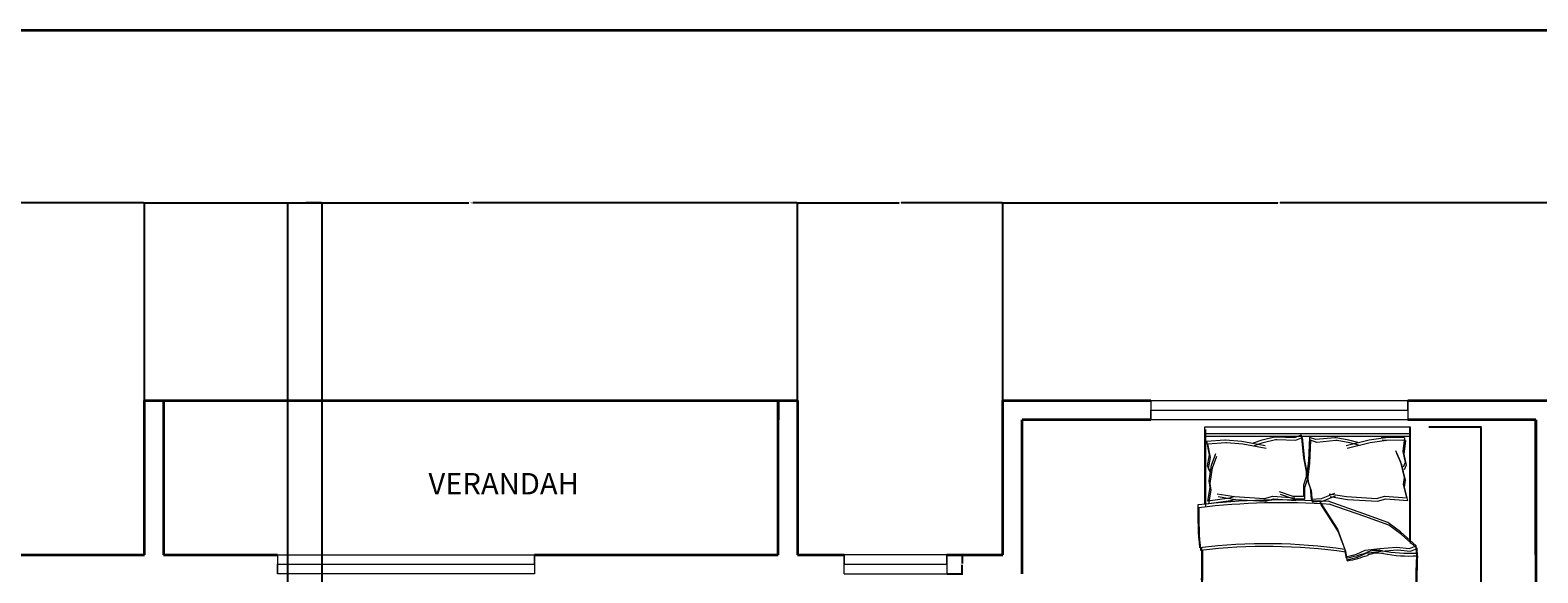
# Model space of a CAD drawing. Units: inches. Extents: x 1937 to 2996, y 1402 to 2323.
# Tile 8 of 10: x 2290 to 2643, y 2197 to 2323. Entities that reach past the tile are written whole.
import ezdxf

# ---------------------------------------------------------------- set-up
doc = ezdxf.new("R2010")
doc.units = ezdxf.units.IN
for name, color, linetype, lineweight in [('A-ANNO-DIMS', 2, 'Continuous', 18), ('A-ANNO-TTLB', 7, 'Continuous', 35), ('A-AREA-IDEN', 7, 'Continuous', 18), ('A-FURN', 8, 'Continuous', 13), ('A-GLAZ', 141, 'Continuous', 18), ('A-WALL', 7, 'Continuous', 35)]:
    doc.layers.add(name, color=color, linetype=linetype, lineweight=lineweight)
doc.styles.get("Standard").update_dxf_attribs({"font": 'arial.ttf'})
doc.dimstyles.get("Standard").update_dxf_attribs({"dimtxt": 0.18, "dimasz": 0.18, "dimexe": 0.18, "dimexo": 0.0625, "dimgap": 0.09, "dimtad": 0, "dimtih": 1, "dimtoh": 1, "dimdec": 4, "dimzin": 0, "dimdsep": 46, "dimtxsty": 'Standard', "dimcen": 0.09, "dimadec": 0, "dimazin": 0, "dimtfac": 1, "dimtdec": 4, "dimtofl": 0, "dimtmove": 0, "dimatfit": 3, "dimfxl": 1, "dimtolj": 1, "dimtzin": 0, "dimarcsym": 0})

# ---------------------------------------------------------------- blocks, each defined once
blk = doc.blocks.new('BED-DOUBLE')
for p, q in [((-24.01, -18.11), (-24.01, 0)), ((-24.01, -18.11), (-24.01, 0)), ((-24.01, 0), (24.01, 0)), ((23.78, 0), (23.78, -26.61)), ((23.78, 0), (23.78, -26.61)), ((24.01, 0), (24.01, -0.64)), ((-24.01, -1.53), (23.78, -1.53)), ((-24.01, -1.53), (23.78, -1.53)), ((-23.78, -18.75), (-23.78, -0.64)), ((-23.78, -18.75), (-23.78, -0.64)), ((-23.78, -2.17), (24.01, -2.17)), ((-23.78, -2.17), (24.01, -2.17)), ((-23.59, -3.34), (-19.3, -3.01)), ((-23.59, -3.34), (-19.31, -3.01)), ((-23.59, -3.32), (-23.01, -6.5)), ((-23.59, -3.32), (-23.01, -6.5)), ((-19.31, -3.01), (-19.2, -3.03)), ((-19.3, -3.01), (-19.2, -3.03)), ((-19.2, -3.03), (-15.38, -3.32)), ((-19.2, -3.03), (-15.38, -3.32)), ((-15.38, -3.32), (-9.88, -4.33)), ((-15.38, -3.32), (-9.88, -4.33)), ((-12.63, -3.75), (-10.61, -3.03)), ((-12.63, -3.75), (-10.61, -3.03)), ((-10.61, -3.03), (-7.71, -2.3)), ((-10.61, -3.03), (-7.71, -2.3)), ((-10.38, -3.67), (-7.49, -2.94)), ((-10.38, -3.67), (-7.49, -2.94)), ((-7.71, -2.3), (-7.39, -2.3)), ((-7.71, -2.3), (-7.39, -2.3)), ((-7.49, -2.94), (-7.16, -2.94)), ((-7.49, -2.94), (-7.16, -2.94)), ((-7.39, -2.3), (-2.95, -2.45)), ((-7.39, -2.3), (-2.95, -2.45)), ((-7.16, -2.94), (-2.72, -3.09)), ((-7.16, -2.94), (-2.72, -3.09)), ((-2.95, -2.45), (-1.5, -1.87)), ((-2.95, -2.45), (-1.5, -1.87)), ((-2.72, -3.09), (-1.27, -2.51)), ((-2.72, -3.09), (-1.27, -2.51)), ((-1.5, -1.87), (-0.92, -7.22)), ((-1.5, -1.87), (-0.92, -7.22)), ((-1.27, -2.51), (-0.7, -7.86)), ((-1.27, -2.51), (-0.7, -7.86)), ((0.49, -2.49), (0.25, -7.87)), ((0.49, -2.49), (0.25, -7.87)), ((0.72, -3.13), (0.48, -8.51)), ((0.72, -3.13), (0.48, -8.51)), ((1.97, -2.98), (0.49, -2.49)), ((1.97, -2.98), (0.49, -2.49)), ((2.2, -3.62), (0.72, -3.13)), ((2.2, -3.62), (0.72, -3.13)), ((6.4, -2.56), (1.97, -2.98)), ((6.4, -2.56), (1.97, -2.98)), ((6.63, -3.2), (2.2, -3.62)), ((6.63, -3.2), (2.2, -3.62)), ((6.72, -2.54), (6.4, -2.56)), ((6.72, -2.54), (6.4, -2.56)), ((6.95, -3.18), (6.63, -3.2)), ((6.95, -3.18), (6.63, -3.2)), ((9.65, -3.08), (6.72, -2.54)), ((9.65, -3.08), (6.72, -2.54)), ((9.88, -3.72), (6.95, -3.18)), ((9.88, -3.72), (6.95, -3.18)), ((14.43, -3.07), (9.01, -4.42)), ((14.43, -3.07), (9.01, -4.42)), ((11.72, -3.67), (9.65, -3.08)), ((11.72, -3.67), (9.65, -3.08)), ((18.23, -2.54), (14.43, -3.07)), ((18.23, -2.54), (14.43, -3.07)), ((18.46, -3.18), (14.66, -3.71)), ((18.46, -3.18), (14.66, -3.71)), ((22.63, -2.56), (17.23, -2.46)), ((17.23, -2.46), (18.23, -2.54)), ((22.63, -2.56), (17.23, -2.46)), ((17.23, -2.46), (18.23, -2.54)), ((22.86, -3.2), (17.45, -3.1)), ((17.45, -3.1), (18.46, -3.18)), ((22.86, -3.2), (17.45, -3.1)), ((17.45, -3.1), (18.46, -3.18)), ((22.63, -2.56), (22.25, -5.77)), ((22.63, -2.56), (22.25, -5.77)), ((22.86, -3.2), (22.48, -6.41)), ((22.86, -3.2), (22.48, -6.41)), ((24.01, -0.64), (24.01, -27.25)), ((24.01, -0.64), (24.01, -27.25)), ((-23.01, -6.5), (-23.45, -9.1)), ((-23.01, -6.5), (-23.45, -9.1)), ((-23.36, -3.98), (-19.08, -3.65)), ((-23.36, -3.98), (-19.08, -3.65)), ((-23.36, -3.96), (-22.78, -7.14)), ((-23.36, -3.96), (-22.78, -7.14)), ((-22.43, -8.96), (-21.42, -6.21)), ((-22.43, -8.96), (-21.42, -6.21)), ((-22.21, -9.59), (-21.19, -6.85)), ((-22.2, -9.59), (-21.19, -6.85)), ((-19.08, -3.65), (-18.97, -3.67)), ((-19.08, -3.65), (-18.97, -3.67)), ((-18.97, -3.67), (-15.15, -3.96)), ((-18.97, -3.67), (-15.15, -3.96)), ((-15.15, -3.96), (-9.65, -4.97)), ((-15.15, -3.96), (-9.65, -4.97)), ((-12.4, -4.39), (-10.38, -3.67)), ((-12.4, -4.39), (-10.38, -3.67)), ((14.66, -3.71), (9.24, -5.06)), ((14.66, -3.71), (9.24, -5.06)), ((11.94, -4.31), (9.88, -3.72)), ((11.94, -4.31), (9.88, -3.72)), ((21.83, -8.26), (20.64, -5.58)), ((21.82, -8.26), (20.64, -5.58)), ((22.05, -8.9), (20.87, -6.22)), ((22.05, -8.9), (20.87, -6.22)), ((22.25, -5.77), (22.84, -8.34)), ((22.25, -5.77), (22.84, -8.34)), ((22.48, -6.41), (23.07, -8.98)), ((22.48, -6.41), (23.07, -8.98)), ((-23.45, -9.1), (-22.87, -10.11)), ((-23.45, -9.1), (-22.87, -10.11)), ((-22.78, -7.14), (-23.22, -9.74)), ((-22.78, -7.14), (-23.22, -9.74)), ((-23.22, -9.74), (-22.64, -10.75)), ((-23.22, -9.74), (-22.64, -10.75)), ((-23.01, -12.57), (-22.43, -8.96)), ((-23.01, -12.57), (-22.43, -8.96)), ((-22.78, -13.21), (-22.2, -9.59)), ((-22.78, -13.21), (-22.21, -9.59)), ((-0.92, -7.22), (-0.35, -10.4)), ((-0.92, -7.22), (-0.35, -10.4)), ((-0.7, -7.86), (-0.12, -11.04)), ((-0.7, -7.86), (-0.12, -11.04)), ((-0.35, -10.4), (-0.35, -11.7)), ((-0.35, -10.4), (-0.35, -11.7)), ((0.25, -7.87), (-0.13, -11.08)), ((0.25, -7.87), (-0.13, -11.08)), ((0.48, -8.51), (0.1, -11.72)), ((0.48, -8.51), (0.1, -11.72)), ((22.63, -11.83), (21.82, -8.26)), ((22.63, -11.83), (21.83, -8.26)), ((22.86, -12.47), (22.05, -8.9)), ((22.86, -12.47), (22.05, -8.9)), ((22.84, -8.34), (22.33, -9.38)), ((22.84, -8.34), (22.33, -9.38)), ((23.07, -8.98), (22.56, -10.02)), ((23.07, -8.98), (22.56, -10.02)), ((-22.72, -14.16), (-23.01, -12.57)), ((-22.72, -14.16), (-23.01, -12.57)), ((-22.49, -14.8), (-22.78, -13.21)), ((-22.49, -14.8), (-22.78, -13.21)), ((-0.35, -11.7), (-0.92, -13.58)), ((-0.35, -11.7), (-0.92, -13.58)), ((-0.92, -13.58), (-0.92, -16.26)), ((-0.92, -13.58), (-0.92, -16.26)), ((-0.12, -12.34), (-0.7, -14.22)), ((-0.12, -12.34), (-0.7, -14.22)), ((-0.13, -11.08), (-0.05, -12.38)), ((-0.13, -11.08), (-0.05, -12.38)), ((-0.12, -11.04), (-0.12, -12.34)), ((-0.12, -11.04), (-0.12, -12.34)), ((-0.05, -12.38), (0.65, -14.22)), ((-0.05, -12.38), (0.65, -14.22)), ((0.1, -11.72), (0.18, -13.02)), ((0.1, -11.72), (0.18, -13.02)), ((0.18, -13.02), (0.87, -14.86)), ((0.18, -13.02), (0.87, -14.86)), ((22.44, -13.43), (22.63, -11.83)), ((22.44, -13.43), (22.63, -11.83)), ((23.21, -16.57), (22.44, -13.43)), ((23.21, -16.57), (22.44, -13.43)), ((22.67, -14.07), (22.86, -12.47)), ((22.67, -14.07), (22.86, -12.47)), ((23.44, -17.21), (22.67, -14.07)), ((23.44, -17.21), (22.67, -14.07)), ((-23.3, -17.34), (-22.72, -14.16)), ((-23.3, -17.34), (-22.72, -14.16)), ((-18.2, -16.62), (-23.3, -17.34)), ((-18.2, -16.62), (-23.3, -17.34)), ((-23.07, -17.98), (-22.49, -14.8)), ((-23.07, -17.98), (-22.49, -14.8)), ((-17.98, -17.26), (-23.07, -17.98)), ((-17.98, -17.26), (-23.07, -17.98)), ((-21.1, -15.63), (-17.07, -16.3)), ((-21.1, -15.63), (-17.07, -16.3)), ((-20.87, -16.27), (-16.84, -16.93)), ((-20.87, -16.27), (-16.84, -16.93)), ((-17.07, -16.3), (-18.2, -16.62)), ((-17.07, -16.3), (-18.2, -16.62)), ((-16.84, -16.93), (-17.98, -17.26)), ((-16.84, -16.93), (-17.98, -17.26)), ((-17.07, -16.3), (-10.06, -16.73)), ((-17.07, -16.3), (-10.06, -16.73)), ((-16.84, -16.93), (-9.83, -17.37)), ((-16.84, -16.93), (-9.83, -17.37)), ((-10.06, -16.73), (-8.1, -16.17)), ((-10.06, -16.73), (-8.1, -16.17)), ((-9.83, -17.37), (-7.87, -16.81)), ((-9.83, -17.37), (-7.87, -16.81)), ((-8.1, -16.17), (-2.97, -16.57)), ((-8.1, -16.17), (-2.97, -16.57)), ((-7.87, -16.81), (-2.74, -17.21)), ((-7.87, -16.81), (-2.74, -17.21)), ((-3.38, -16.26), (-6.53, -15.17)), ((-3.38, -16.26), (-6.53, -15.17)), ((-3.15, -16.9), (-6.3, -15.81)), ((-3.15, -16.9), (-6.3, -15.81)), ((-0.92, -16.26), (-3.38, -16.26)), ((-0.92, -16.26), (-3.38, -16.26)), ((-0.7, -16.9), (-3.15, -16.9)), ((-0.7, -16.9), (-3.15, -16.9)), ((-0.7, -14.22), (-0.7, -16.9)), ((-0.7, -14.22), (-0.7, -16.9)), ((0.65, -14.22), (0.81, -16.89)), ((0.65, -14.22), (0.81, -16.89)), ((0.81, -16.89), (3.27, -16.74)), ((0.81, -16.89), (3.27, -16.74)), ((0.87, -14.86), (1.04, -17.53)), ((0.87, -14.86), (1.04, -17.53)), ((1.04, -17.53), (3.49, -17.38)), ((1.04, -17.53), (3.49, -17.38)), ((2.77, -17.38), (6.97, -23.88)), ((2.77, -17.38), (6.96, -23.88)), ((3.27, -16.74), (6.34, -15.45)), ((3.27, -16.74), (6.34, -15.45)), ((3.49, -17.38), (6.56, -16.09)), ((3.49, -17.38), (6.56, -16.09)), ((13.16, -20.32), (4.82, -17.38)), ((13.16, -20.32), (4.82, -17.38)), ((5.08, -15.63), (9.11, -16.3)), ((5.08, -15.63), (9.11, -16.3)), ((5.31, -16.27), (9.34, -16.93)), ((5.31, -16.27), (9.34, -16.93)), ((9.11, -16.3), (16.12, -16.73)), ((9.11, -16.3), (16.12, -16.73)), ((9.34, -16.93), (16.35, -17.37)), ((9.34, -16.93), (16.35, -17.37)), ((16.12, -16.73), (18.08, -16.17)), ((16.12, -16.73), (18.08, -16.17)), ((16.35, -17.37), (18.31, -16.81)), ((16.35, -17.37), (18.31, -16.81)), ((18.08, -16.17), (23.21, -16.57)), ((18.08, -16.17), (23.21, -16.57)), ((18.31, -16.81), (23.44, -17.21)), ((18.31, -16.81), (23.44, -17.21)), ((3, -18.02), (7.19, -24.52)), ((3, -18.02), (7.19, -24.52)), ((13.39, -20.96), (5.05, -18.02)), ((13.39, -20.96), (5.05, -18.02)), ((18.74, -22.33), (13.16, -20.32)), ((18.74, -22.33), (13.16, -20.32)), ((18.96, -22.97), (13.39, -20.96)), ((18.96, -22.97), (13.39, -20.96)), ((6.96, -23.88), (8.67, -28.37)), ((6.97, -23.88), (8.67, -28.37)), ((7.19, -24.52), (8.9, -29)), ((7.19, -24.52), (8.9, -29)), ((21.68, -24.5), (18.74, -22.33)), ((21.68, -24.5), (18.74, -22.33)), ((21.91, -25.13), (18.96, -22.97)), ((21.91, -25.13), (18.96, -22.97)), ((25.38, -27.75), (21.68, -24.5)), ((25.38, -27.75), (21.68, -24.5)), ((16.88, -28.37), (20.75, -28.06)), ((16.88, -28.37), (20.75, -28.06)), ((20.75, -28.06), (23.85, -28.37)), ((20.75, -28.06), (23.85, -28.37)), ((25.61, -28.39), (21.91, -25.13)), ((25.61, -28.39), (21.91, -25.13)), ((23.85, -28.37), (25.38, -27.75)), ((23.85, -28.37), (25.38, -27.75)), ((25.46, -29.49), (25.38, -27.75, 3.87)), ((25.46, -29.49), (25.38, -27.75, 3.87)), ((8.67, -28.37), (8.98, -30.38)), ((8.67, -28.37), (8.98, -30.38)), ((8.9, -29), (9.21, -31.02)), ((8.9, -29), (9.21, -31.02)), ((8.98, -30.38), (11.46, -29.76)), ((8.98, -30.38), (11.46, -29.76)), ((9.21, -31.02), (11.68, -30.4)), ((9.21, -31.02), (11.68, -30.4)), ((11.46, -29.76), (13.47, -28.83)), ((11.46, -29.76), (13.47, -28.83)), ((11.68, -30.4), (13.7, -29.47)), ((11.68, -30.4), (13.7, -29.47)), ((13.47, -28.83), (16.88, -28.37)), ((13.47, -28.83), (16.88, -28.37)), ((13.7, -29.47), (17.11, -29)), ((13.7, -29.47), (17.1, -29)), ((17.1, -29), (20.98, -28.69)), ((17.11, -29), (20.98, -28.69)), ((20.98, -28.69), (24.07, -29)), ((20.98, -28.69), (24.07, -29)), ((24.07, -29), (25.61, -28.39)), ((24.07, -29), (25.61, -28.39)), ((25.69, -30.13), (25.61, -28.39, 3.87)), ((25.69, -30.13), (25.61, -28.39, 3.87)), ((-12.42, -79.25), (12.19, -79.25)), ((-12.42, -79.25), (12.19, -79.25)), ((-12.19, -79.88), (12.42, -79.88)), ((-12.19, -79.88), (12.42, -79.88))]:
    blk.add_line(p, q)
for centre, radius, start, end in [((-6.13, -182.05), 164.97, 86.0865, 96.7821), ((-6.13, -182.05), 164.97, 86.0865, 96.7821), ((57.68, -20.1), 83.31, 178.7218, 185.604), ((57.68, -20.1), 83.31, 178.7218, 185.604), ((57.91, -20.74), 83.31, 178.7218, 185.604), ((57.91, -20.74), 83.31, 178.7218, 185.604), ((-5.9, -182.69), 164.97, 86.0865, 96.7821), ((-5.9, -182.69), 164.97, 86.0865, 96.7821), ((-9.73, -156.32), 129.02, 81.7845, 96.9006), ((-9.73, -156.32), 129.02, 81.7845, 96.9006), ((-9.5, -156.96), 129.02, 81.7845, 96.9006), ((-9.5, -156.96), 129.02, 81.7845, 96.9006), ((-194.79, -31.17), 170.11, 358.4762, 1.0082), ((-194.79, -31.17), 170.11, 358.4762, 1.0082), ((-194.56, -31.81), 170.11, 358.4762, 1.0082), ((-194.56, -31.81), 170.11, 358.4762, 1.0082), ((9.15, -30.44), 0.185, 160.2464, 271.1377), ((9.15, -30.44), 0.185, 160.2464, 271.1377), ((3.67, -1.48), 29.65, 280.6617, 289.8806), ((3.67, -1.48), 29.65, 280.6617, 289.8806), ((9.38, -31.08), 0.185, 160.2464, 271.1377), ((9.38, -31.08), 0.185, 160.2464, 271.1377), ((3.9, -2.12), 29.65, 280.6617, 289.8806), ((3.9, -2.12), 29.65, 280.6617, 289.8806), ((16.26, -35.07), 6.22, 78.6608, 113.7384), ((16.26, -35.07), 6.22, 78.6608, 113.7384), ((16.49, -35.71), 6.22, 78.6608, 113.7384), ((16.49, -35.71), 6.22, 78.6608, 113.7384), ((23.84, 6.66), 36.18, 259.8763, 272.5657), ((23.84, 6.66), 36.18, 259.8763, 272.5657), ((24.07, 6.02), 36.18, 259.8763, 272.5657), ((24.07, 6.02), 36.18, 259.8763, 272.5657), ((154.78, -36.32), 129.5, 176.9791, 183.8365), ((154.78, -36.32), 129.5, 176.9791, 183.8365), ((155.01, -36.95), 129.5, 176.9791, 183.8365), ((155.01, -36.95), 129.5, 176.9791, 183.8365), ((457.34, -50.61), 482.31, 178.2277, 181.7185), ((457.34, -50.61), 482.31, 178.2277, 181.7185), ((457.57, -51.25), 482.31, 178.2277, 181.7185), ((457.57, -51.25), 482.31, 178.2277, 181.7185), ((-4536.23, -67.82), 4561.86, 0.00217, 0.28689), ((-4536.23, -67.82), 4561.86, 0.00217, 0.28689), ((-4536, -68.46), 4561.86, 0.00217, 0.28689), ((-4536, -68.46), 4561.86, 0.00217, 0.28689), ((-54.38, -64.52), 29.63, 346.0648, 358.9113), ((-54.38, -64.52), 29.63, 346.0648, 358.9113), ((-54.16, -65.15), 29.63, 346.0648, 358.9113), ((-54.16, -65.15), 29.63, 346.0648, 358.9113), ((48.67, -68.67), 23.07, 177.4714, 206.4681), ((48.67, -68.67), 23.07, 177.4714, 206.4681), ((48.9, -69.31), 23.07, 177.4714, 206.4681), ((48.9, -69.31), 23.07, 177.4714, 206.4681), ((-49.14, -70.28), 23.56, 337.9751, 356.652), ((-49.14, -70.28), 23.56, 337.9751, 356.652), ((-48.92, -70.91), 23.56, 337.9751, 356.652), ((-48.92, -70.91), 23.56, 337.9751, 356.652), ((-26.4, -79.72), 1.09, 146.1736, 293.4781), ((-26.4, -79.72), 1.09, 146.1736, 293.4781), ((-26.17, -80.36), 1.09, 146.1736, 293.4781), ((-26.17, -80.36), 1.09, 146.1736, 293.4781), ((-6.06, -200.84), 121.76, 92.9958, 99.4091), ((-6.06, -200.84), 121.76, 92.9958, 99.4091), ((-5.83, -201.48), 121.76, 92.9958, 99.4091), ((-5.83, -201.48), 121.76, 92.9958, 99.4091), ((-44.71, 23.71), 106.46, 283.3832, 287.7053), ((-44.71, 23.71), 106.46, 283.3832, 287.7053), ((-44.48, 23.07), 106.46, 283.3832, 287.7053), ((-44.48, 23.07), 106.46, 283.3832, 287.7053), ((13.67, -212.28), 133.04, 84.4998, 90.6351), ((13.67, -212.28), 133.04, 84.4998, 90.6351), ((13.9, -212.92), 133.04, 84.4998, 90.6351), ((13.9, -212.92), 133.04, 84.4998, 90.6351), ((26.93, -78.87), 1.1, 242.6588, 356.02), ((26.93, -78.87), 1.1, 242.6588, 356.02), ((27.15, -79.51), 1.1, 242.6588, 356.02), ((27.15, -79.51), 1.1, 242.6588, 356.02)]:
    blk.add_arc(centre, radius, start, end)
blk = doc.blocks.new('WINDOW-60IN')
for p, q in [((0, 2.25), (0, -2.25)), ((0, 2.25), (60, 2.25)), ((0, -2.25), (0, 0)), ((0, 0), (60, 0)), ((60, 0), (60, 2.25)), ((60, 2.25), (60, -2.25)), ((60, -2.25), (0, -2.25))]:
    blk.add_line(p, q)
blk = doc.blocks.new('WINDOW-24IN-JAMB-B')
for p, q in [((0, -2.25), (0, 2.25)), ((0, 2.25), (0, 0)), ((24, 2.25), (0, 2.25)), ((0, 0), (24, 0)), ((24, 0), (24, 2.25)), ((24, 2.25), (24, -2.25)), ((0, -2.25), (24, -2.25))]:
    blk.add_line(p, q)
blk = doc.blocks.new('*D9')
at = {"layer": 'A-ANNO-DIMS', "color": 0, "lineweight": -2, "transparency": 16777216}
for p, q in [((2617.12, 2230.66), (2629.47, 2230.66)), ((2629.29, 2230.48), (2629.29, 2190.07)), ((2629.29, 2149.29), (2629.29, 2189.7)), ((2617.12, 2149.11), (2629.47, 2149.11))]:
    blk.add_line(p, q, dxfattribs=at)
at = {"layer": 'A-ANNO-DIMS', "color": 0, "transparency": 16777216}
for points in [[(2629.26, 2230.48), (2629.32, 2230.48), (2629.29, 2230.66)], [(2629.26, 2149.29), (2629.32, 2149.29), (2629.29, 2149.11)]]:
    blk.add_solid(points, dxfattribs=at)
at = {"layer": 'Defpoints', "color": 0, "transparency": 16777216}
for p in [(2617.06, 2230.66), (2629.29, 2230.66), (2617.06, 2149.11)]:
    blk.add_point(p, dxfattribs=at)
at = {"layer": 'A-ANNO-DIMS', "color": 0, "transparency": 16777216, "insert": (2629.29, 2189.88), "char_height": 0.18, "attachment_point": 5}
blk.add_mtext('\\A1;DOUBLE BED 82 TYP.', dxfattribs=at)
blk = doc.blocks.new('*D18')
at = {"layer": 'A-ANNO-DIMS', "color": 0, "lineweight": -2, "transparency": 16777216}
for p, q in [((2504.58, 2200.81), (2508.3, 2200.81)), ((2508.12, 2200.63), (2508.12, 2198.74)), ((2508.12, 2196.49), (2508.12, 2198.37)), ((2504.58, 2196.31), (2508.3, 2196.31))]:
    blk.add_line(p, q, dxfattribs=at)
at = {"layer": 'A-ANNO-DIMS', "color": 0, "transparency": 16777216}
for points in [[(2508.09, 2200.63), (2508.15, 2200.63), (2508.12, 2200.81)], [(2508.09, 2196.49), (2508.15, 2196.49), (2508.12, 2196.31)]]:
    blk.add_solid(points, dxfattribs=at)
at = {"layer": 'Defpoints', "color": 0, "transparency": 16777216}
for p in [(2504.52, 2200.81), (2508.12, 2200.81), (2504.52, 2196.31)]:
    blk.add_point(p, dxfattribs=at)
at = {"layer": 'A-ANNO-DIMS', "color": 0, "transparency": 16777216, "insert": (2508.12, 2198.56), "char_height": 0.18, "attachment_point": 5}
blk.add_mtext('\\A1;5 TYP.', dxfattribs=at)
blk = doc.blocks.new('*D26')
at = {"layer": 'A-ANNO-DIMS', "color": 0, "lineweight": -2, "transparency": 16777216}
for p, q in [((2175.65, 2236.87), (2175.65, 2283.14)), ((2175.83, 2282.96), (2245.91, 2282.96)), ((2316.9, 2282.96), (2246.82, 2282.96)), ((2317.08, 2236.87), (2317.08, 2283.14))]:
    blk.add_line(p, q, dxfattribs=at)
at = {"layer": 'A-ANNO-DIMS', "color": 0, "transparency": 16777216}
for points in [[(2175.83, 2282.99), (2175.83, 2282.93), (2175.65, 2282.96)], [(2316.9, 2282.99), (2316.9, 2282.93), (2317.08, 2282.96)]]:
    blk.add_solid(points, dxfattribs=at)
at = {"layer": 'Defpoints', "color": 0, "transparency": 16777216}
for p in [(2317.08, 2282.96), (2175.65, 2236.81), (2317.08, 2236.81)]:
    blk.add_point(p, dxfattribs=at)
at = {"layer": 'A-ANNO-DIMS', "color": 0, "transparency": 16777216, "insert": (2246.36, 2282.96), "char_height": 0.18, "attachment_point": 5}
blk.add_mtext('\\A1;141.43', dxfattribs=at)
blk = doc.blocks.new('*D27')
at = {"layer": 'A-ANNO-DIMS', "color": 0, "lineweight": -2, "transparency": 16777216}
for p, q in [((2317.08, 2236.87), (2317.08, 2283.14)), ((2317.26, 2282.96), (2392.91, 2282.96)), ((2469.47, 2282.96), (2393.82, 2282.96)), ((2469.65, 2236.87), (2469.65, 2283.14))]:
    blk.add_line(p, q, dxfattribs=at)
at = {"layer": 'A-ANNO-DIMS', "color": 0, "transparency": 16777216}
for points in [[(2317.26, 2282.99), (2317.26, 2282.93), (2317.08, 2282.96)], [(2469.47, 2282.99), (2469.47, 2282.93), (2469.65, 2282.96)]]:
    blk.add_solid(points, dxfattribs=at)
at = {"layer": 'Defpoints', "color": 0, "transparency": 16777216}
for p in [(2469.65, 2282.96), (2317.08, 2236.81), (2469.65, 2236.81)]:
    blk.add_point(p, dxfattribs=at)
at = {"layer": 'A-ANNO-DIMS', "color": 0, "transparency": 16777216, "insert": (2393.36, 2282.96), "char_height": 0.18, "attachment_point": 5}
blk.add_mtext('\\A1;152.57', dxfattribs=at)
blk = doc.blocks.new('*D28')
at = {"layer": 'A-ANNO-DIMS', "color": 0, "lineweight": -2, "transparency": 16777216}
for p, q in [((2469.65, 2236.87), (2469.65, 2283.14)), ((2469.83, 2282.96), (2493.42, 2282.96)), ((2517.47, 2282.96), (2493.87, 2282.96)), ((2517.65, 2236.87), (2517.65, 2283.14))]:
    blk.add_line(p, q, dxfattribs=at)
at = {"layer": 'A-ANNO-DIMS', "color": 0, "transparency": 16777216}
for points in [[(2469.83, 2282.99), (2469.83, 2282.93), (2469.65, 2282.96)], [(2517.47, 2282.99), (2517.47, 2282.93), (2517.65, 2282.96)]]:
    blk.add_solid(points, dxfattribs=at)
at = {"layer": 'Defpoints', "color": 0, "transparency": 16777216}
for p in [(2517.65, 2282.96), (2469.65, 2236.81), (2517.65, 2236.81)]:
    blk.add_point(p, dxfattribs=at)
at = {"layer": 'A-ANNO-DIMS', "color": 0, "transparency": 16777216, "insert": (2493.65, 2282.96), "char_height": 0.18, "attachment_point": 5}
blk.add_mtext('\\A1;48', dxfattribs=at)
blk = doc.blocks.new('*D29')
at = {"layer": 'A-ANNO-DIMS', "color": 0, "lineweight": -2, "transparency": 16777216}
for p, q in [((2517.65, 2236.87), (2517.65, 2283.14)), ((2517.83, 2282.96), (2581.87, 2282.96)), ((2646.47, 2282.96), (2582.43, 2282.96)), ((2646.65, 2236.87), (2646.65, 2283.14))]:
    blk.add_line(p, q, dxfattribs=at)
at = {"layer": 'A-ANNO-DIMS', "color": 0, "transparency": 16777216}
for points in [[(2517.83, 2282.99), (2517.83, 2282.93), (2517.65, 2282.96)], [(2646.47, 2282.99), (2646.47, 2282.93), (2646.65, 2282.96)]]:
    blk.add_solid(points, dxfattribs=at)
at = {"layer": 'Defpoints', "color": 0, "transparency": 16777216}
for p in [(2646.65, 2282.96), (2517.65, 2236.81), (2646.65, 2236.81)]:
    blk.add_point(p, dxfattribs=at)
at = {"layer": 'A-ANNO-DIMS', "color": 0, "transparency": 16777216, "insert": (2582.15, 2282.96), "char_height": 0.18, "attachment_point": 5}
blk.add_mtext('\\A1;129', dxfattribs=at)
blk = doc.blocks.new('*D36')
at = {"layer": 'A-ANNO-DIMS', "color": 0, "lineweight": -2, "transparency": 16777216}
for p, q in [((2350.61, 1896.12), (2350.61, 2283.14)), ((2350.79, 2282.96), (2354.46, 2282.96)), ((2358.43, 2282.96), (2354.76, 2282.96)), ((2358.61, 1896.12), (2358.61, 2283.14))]:
    blk.add_line(p, q, dxfattribs=at)
at = {"layer": 'A-ANNO-DIMS', "color": 0, "transparency": 16777216}
for points in [[(2350.79, 2282.99), (2350.79, 2282.93), (2350.61, 2282.96)], [(2358.43, 2282.99), (2358.43, 2282.93), (2358.61, 2282.96)]]:
    blk.add_solid(points, dxfattribs=at)
at = {"layer": 'Defpoints', "color": 0, "transparency": 16777216}
for p in [(2358.61, 2282.96), (2350.61, 1896.06), (2358.61, 1896.06)]:
    blk.add_point(p, dxfattribs=at)
at = {"layer": 'A-ANNO-DIMS', "color": 0, "transparency": 16777216, "insert": (2354.61, 2282.96), "char_height": 0.18, "attachment_point": 5}
blk.add_mtext('\\A1;8', dxfattribs=at)

msp = doc.modelspace()

# ---------------------------------------------------------------- linework, layer by layer
at = {"layer": 'A-ANNO-TTLB'}
msp.add_lwpolyline([(1937.1125, 2323.2883), (2995.8132, 2323.2883), (2995.8132, 1401.6335), (1937.1125, 1401.6335)], close=True, dxfattribs=at)
at = {"layer": 'A-WALL'}
for p, q in [((2317.081, 2200.8061), (2317.081, 2236.8061)), ((2317.081, 2236.8061), (2469.6473, 2236.8061)), ((2321.581, 2236.8061), (2321.581, 2200.8061)), ((2465.1473, 2200.8061), (2465.1473, 2236.8061)), ((2465.1473, 2236.8061), (2465.1473, 2232.3061)), ((2469.6473, 2236.8061), (2469.6473, 2200.8061)), ((2517.6473, 2200.8061), (2517.6473, 2236.8061)), ((2517.6473, 2236.8061), (2552.1965, 2236.8061)), ((2612.1965, 2236.8061), (2646.6473, 2236.8061)), ((2522.1473, 2200.8061), (2522.1473, 2232.3061)), ((2552.1965, 2232.3061), (2522.1473, 2232.3061)), ((2642.1473, 2232.3061), (2612.1965, 2232.3061)), ((2642.1473, 2232.3061), (2642.1473, 2070.3061)), ((2642.1473, 2200.8061), (2642.1473, 2232.3061)), ((2276.3117, 2200.8061), (2317.081, 2200.8061)), ((2321.581, 2200.8061), (2348.1952, 2200.8061)), ((2408.1952, 2200.8061), (2465.1473, 2200.8061)), ((2469.6473, 2200.8061), (2480.5154, 2200.8061)), ((2504.5154, 2200.8061), (2517.6473, 2200.8061)), ((2522.1473, 2196.3061), (2522.1473, 2200.8061))]:
    msp.add_line(p, q, dxfattribs=at)

# ---------------------------------------------------------------- block references
at = {"layer": 'A-FURN'}
msp.add_blockref('BED-DOUBLE', (2588.8017, 2230.6586), dxfattribs=at)
at = {"layer": 'A-GLAZ'}
for name, p in [('WINDOW-60IN', (2552.1965, 2234.5561)), ('WINDOW-60IN', (2348.1952, 2198.5561)), ('WINDOW-24IN-JAMB-B', (2480.5154, 2198.5561))]:
    msp.add_blockref(name, p, dxfattribs=at)

# ---------------------------------------------------------------- texts
at = {"layer": 'A-AREA-IDEN', "insert": (2383.4357, 2219.8875), "char_height": 5, "attachment_point": 1}
msp.add_mtext_dynamic_manual_height_columns('VERANDAH', width=137.071433, gutter_width=12.5, heights=[0], dxfattribs=at)

# ---------------------------------------------------------------- dimensions: what is measured, and where the dimension line sits
at = {"layer": 'A-ANNO-DIMS'}
for base, p1, p2, override, picture, middle in [((2317.081, 2282.9561), (2175.6473, 2236.8061), (2317.081, 2236.8061), {"dimdec": 2, "dimlfac": 1, "dimrnd": 0, "dimzin": 0, "dimdsep": 46, "dimlunit": 2}, '*D26', (2246.3642, 2282.9561)), ((2469.6473, 2282.9561), (2317.081, 2236.8061), (2469.6473, 2236.8061), {"dimdec": 2, "dimlfac": 1, "dimrnd": 0, "dimzin": 0, "dimdsep": 46, "dimlunit": 2}, '*D27', (2393.3642, 2282.9561)), ((2358.6104, 2282.9561), (2350.6104, 1896.0561), (2358.6104, 1896.0561), {"dimdec": 0, "dimlfac": 1, "dimrnd": 0, "dimzin": 0, "dimdsep": 46, "dimlunit": 2}, '*D36', (2354.6104, 2282.9561)), ((2517.6473, 2282.9561), (2469.6473, 2236.8061), (2517.6473, 2236.8061), {"dimdec": 0, "dimlfac": 1, "dimrnd": 0, "dimzin": 0, "dimdsep": 46, "dimlunit": 2}, '*D28', (2493.6473, 2282.9561)), ((2646.6473, 2282.9561), (2517.6473, 2236.8061), (2646.6473, 2236.8061), {"dimdec": 0, "dimlfac": 1, "dimrnd": 0, "dimzin": 0, "dimdsep": 46, "dimlunit": 2}, '*D29', (2582.1473, 2282.9561))]:
    dim = msp.add_linear_dim(base=base, p1=p1, p2=p2, dimstyle='Standard', override=override, dxfattribs=at)
    dim.commit()
    dim.dimension.update_dxf_attribs({"geometry": picture, "text_midpoint": middle})
for base, p1, p2, text, picture, middle in [((2629.2877, 2230.6586), (2617.0554, 2149.11), (2617.0554, 2230.6586), 'DOUBLE BED <> TYP.', '*D9', (2629.2877, 2189.8843)), ((2508.1154072539, 2200.8061190364), (2504.5154072539, 2196.3061190364), (2504.5154072539, 2200.8061190364), '<> TYP.', '*D18', (2508.1154072539, 2198.5561190364))]:
    dim = msp.add_linear_dim(base=base, p1=p1, p2=p2, angle=90, text=text, dimstyle='Standard', override={"dimdec": 0, "dimlfac": 1, "dimrnd": 0, "dimzin": 0, "dimdsep": 46, "dimlunit": 2}, dxfattribs=at)
    dim.commit()
    dim.dimension.update_dxf_attribs({"geometry": picture, "text_midpoint": middle})

doc.saveas('drawing.dxf')
